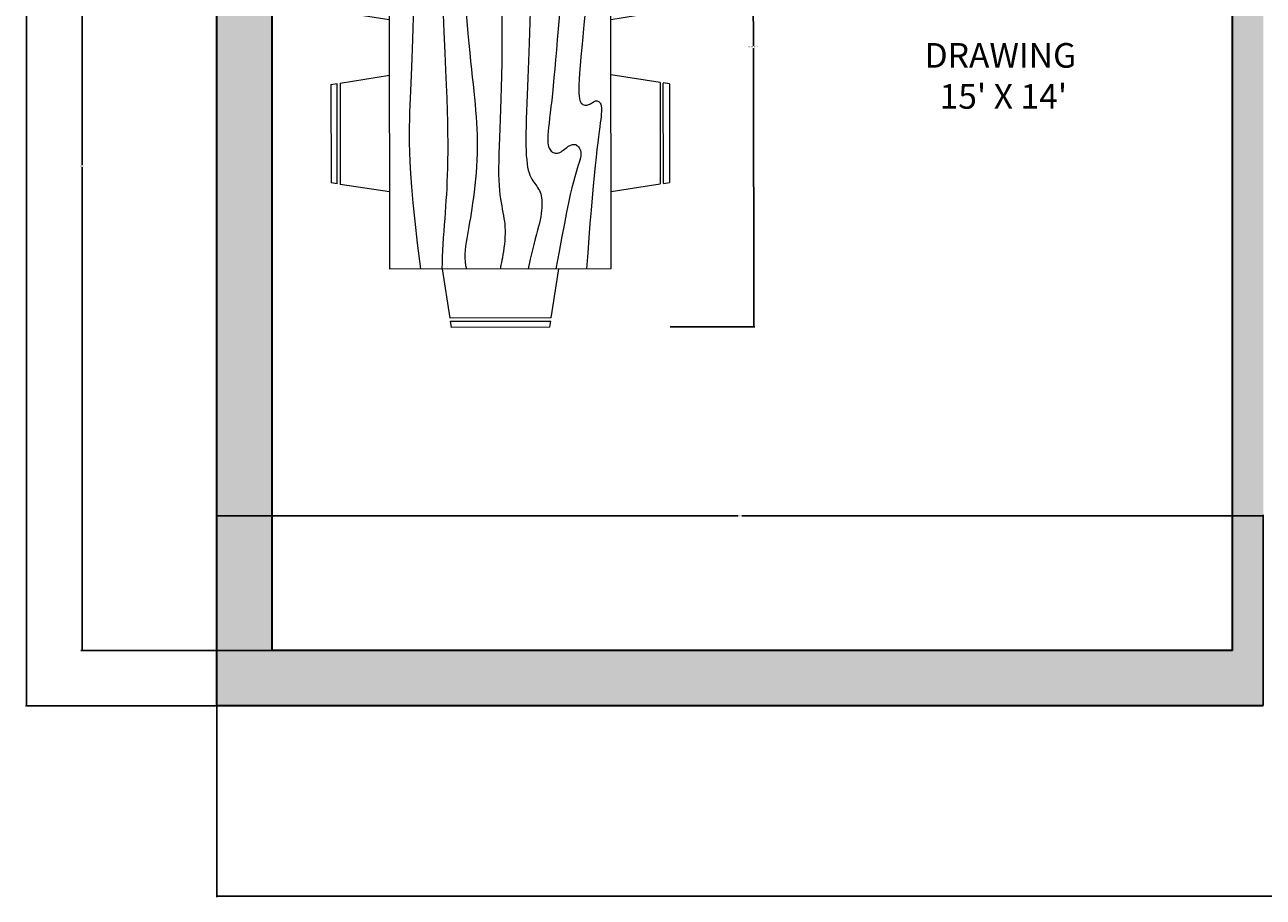
# Model space of a CAD drawing. Units: inches. Extents: x -30 to 437, y -29 to 647.
# Tile 1 of 15: x -30 to 172, y -29 to 113. Entities that reach past the tile are written whole.
import ezdxf

# ---------------------------------------------------------------- set-up
doc = ezdxf.new("R2010")
doc.units = ezdxf.units.IN
doc.header["$MEASUREMENT"] = 0
for name, color, linetype, lineweight in [('A-ANNO-DIMS', 2, 'Continuous', 18), ('A-AREA-IDEN', 7, 'Continuous', 18), ('A-WALL', 7, 'Continuous', 35), ('furniture', 220, 'Continuous', 18)]:
    doc.layers.add(name, color=color, linetype=linetype, lineweight=lineweight)
doc.layers.add('A-WALL-PATT', color=251, linetype='Continuous', lineweight=13, true_color=0x636466)
doc.styles.get("Standard").update_dxf_attribs({"font": 'arial.ttf'})
doc.dimstyles.get("Standard").update_dxf_attribs({"dimtxt": 0.18, "dimasz": 0.18, "dimexe": 0.18, "dimexo": 0.0625, "dimgap": 0.09, "dimtad": 0, "dimtih": 1, "dimtoh": 1, "dimdec": 4, "dimzin": 0, "dimdsep": 46, "dimtxsty": 'Standard', "dimcen": 0.09, "dimadec": 0, "dimazin": 0, "dimtfac": 1, "dimtdec": 4, "dimtofl": 0, "dimtmove": 0, "dimatfit": 3, "dimfxl": 1, "dimtolj": 1, "dimtzin": 0, "dimarcsym": 0})

# ---------------------------------------------------------------- blocks, each defined once
blk = doc.blocks.new('Dining Set - 36 x 72 in.')
for p, q in [((-22, 27.5), (-22.1562, 26.50042)), ((-5.8416, 26.5), (-22.1534, 26.5)), ((-22, 27.5), (-6, 27.5)), ((-5.8437, 26.49966), (-6, 27.5)), ((6, 27.5), (5.8438, 26.50042)), ((22.1584, 26.5), (5.8466, 26.5)), ((6, 27.5), (22, 27.5)), ((22.1563, 26.49966), (22, 27.5)), ((-22.2343, 26.00059), (-23.4847, 17.99762)), ((-22.2304, 26), (-5.7608, 26)), ((-4.5152, 17.99762), (-5.7655, 25.99926)), ((5.7657, 26.00059), (4.5153, 17.99762)), ((5.7696, 26), (22.2392, 26)), ((23.4848, 17.99762), (22.2345, 25.99926)), ((36, 18), (-36, 18)), ((-36, 18), (-36, -18)), ((36, -18), (36, 18)), ((-45.5, 8), (-44.5004, 8.15617)), ((-44.5, -8.15843), (-44.5, 8.15338)), ((-44.0006, 8.23428), (-35.9976, 9.48474)), ((-44, 8.23041), (-44, -8.23915)), ((44.0006, 8.23428), (35.9976, 9.48474)), ((44, 8.23041), (44, -8.23915)), ((44.5, -8.15843), (44.5, 8.15338)), ((45.5, 8), (44.5005, 8.15617)), ((-45.5, 8), (-45.5, -8)), ((45.5, 8), (45.5, -8)), ((-44.4997, -8.15631), (-45.5, -8)), ((44.4997, -8.15631), (45.5, -8)), ((-35.9976, -9.48476), (-43.9993, -8.2345)), ((35.9976, -9.48476), (43.9993, -8.2345)), ((-36, -18), (36, -18)), ((-22.2343, -26.0006), (-23.4847, -17.99762)), ((-4.5152, -17.99762), (-5.7655, -25.99928)), ((5.7657, -26.0006), (4.5153, -17.99762)), ((23.4848, -17.99762), (22.2345, -25.99928)), ((-22.2304, -26), (-5.7608, -26)), ((5.7696, -26), (22.2392, -26)), ((-22, -27.5), (-22.1562, -26.50044)), ((-5.8416, -26.5), (-22.1534, -26.5)), ((-22, -27.5), (-6, -27.5)), ((-5.8437, -26.49967), (-6, -27.5)), ((6, -27.5), (5.8438, -26.50044)), ((22.1584, -26.5), (5.8466, -26.5)), ((6, -27.5), (22, -27.5)), ((22.1563, -26.49967), (22, -27.5))]:
    blk.add_line(p, q)
for points in [[(-36, 15), (-31.1772, 14.97754), (-26.8079, 14.91406), (-22.8538, 14.81543), (-19.276, 14.6875), (-16.0362, 14.53613), (-13.0957, 14.36718), (-10.4159, 14.18652), (-7.9583, 14), (-5.6904, 13.81315), (-3.6035, 13.63021), (-1.6954, 13.45508), (0.0365, 13.29166), (1.5945, 13.14388), (2.9811, 13.01562), (4.1988, 12.9108), (5.25, 12.83333), (6.1393, 12.78613), (6.8802, 12.76823), (7.4883, 12.77767), (7.9792, 12.8125), (8.3685, 12.87077), (8.6719, 12.95052), (8.9049, 13.0498), (9.0833, 13.16666), (9.2205, 13.29899), (9.3216, 13.44401), (9.3895, 13.59879), (9.4271, 13.76041), (9.4373, 13.92594), (9.4232, 14.09245), (9.3875, 14.257), (9.3333, 14.41666), (9.2638, 14.56917), (9.1836, 14.71484), (9.0975, 14.85465), (9.0104, 14.98958), (8.9272, 15.1206), (8.8529, 15.2487), (8.7922, 15.37483), (8.75, 15.5), (8.7305, 15.62467), (8.7344, 15.74739), (8.7617, 15.86621), (8.8125, 15.97916), (8.8867, 16.08431), (8.9844, 16.17968), (9.1055, 16.26334), (9.25, 16.33333), (9.4189, 16.38802), (9.6172, 16.42708), (9.8506, 16.45052), (10.125, 16.45833), (10.4463, 16.45052), (10.8203, 16.42708), (11.2529, 16.38802), (11.75, 16.33333), (12.3184, 16.26318), (12.9694, 16.17838), (13.7151, 16.07991), (14.5677, 15.96875), (15.5395, 15.84586), (16.6426, 15.71224), (17.8893, 15.56884), (19.2917, 15.41666), (20.859, 15.25667), (22.5879, 15.08984), (24.4721, 14.91715), (26.5052, 14.73958), (28.6809, 14.5581), (30.9929, 14.3737), (33.4347, 14.18733), (36, 14)], [(-36, 10), (-28.9766, 10.14274), (-23.1725, 10.20442), (-18.4241, 10.19775), (-14.5677, 10.13541), (-11.4399, 10.03011), (-8.877, 9.89453), (-6.7154, 9.74137), (-4.7917, 9.58333), (-2.9698, 9.43082), (-1.2246, 9.28515), (0.4415, 9.14534), (2.026, 9.01041), (3.5266, 8.87939), (4.9408, 8.7513), (6.266, 8.62516), (7.5, 8.5), (8.6411, 8.37549), (9.6914, 8.2539), (10.6538, 8.13818), (11.5312, 8.03125), (12.3267, 7.93603), (13.043, 7.85547), (13.6831, 7.79248), (14.25, 7.75), (14.7471, 7.7303), (15.1797, 7.73307), (15.5537, 7.75732), (15.875, 7.80208), (16.1494, 7.86637), (16.3828, 7.94922), (16.5811, 8.04964), (16.75, 8.16666), (16.8944, 8.29915), (17.0143, 8.44531), (17.1089, 8.60319), (17.1771, 8.77083), (17.218, 8.94629), (17.2305, 9.1276), (17.2137, 9.31282), (17.1667, 9.5), (17.0895, 9.6875), (16.987, 9.875), (16.8649, 10.0625), (16.7292, 10.25), (16.5856, 10.4375), (16.4401, 10.625), (16.2985, 10.8125), (16.1667, 11), (16.05, 11.18733), (15.9518, 11.3737), (15.8752, 11.5581), (15.8229, 11.73958), (15.798, 11.91715), (15.8034, 12.08984), (15.842, 12.25667), (15.9167, 12.41666), (16.0295, 12.56836), (16.1784, 12.70833), (16.3605, 12.83268), (16.5729, 12.9375), (16.8127, 13.01888), (17.0768, 13.07291), (17.3625, 13.0957), (17.6667, 13.08333), (17.9894, 13.03312), (18.3418, 12.94726), (18.7382, 12.82918), (19.1927, 12.68229), (19.7195, 12.51001), (20.3327, 12.31575), (21.0465, 12.10294), (21.875, 11.875), (22.8357, 11.63354), (23.959, 11.37304), (25.2786, 11.08618), (26.8282, 10.76562), (28.6414, 10.40405), (30.752, 9.99414), (33.1936, 9.52856), (36, 9)], [(-36, 5.5), (-30.7157, 5.3348), (-26.069, 5.20963), (-21.9946, 5.11767), (-18.4271, 5.05208), (-15.3009, 5.00602), (-12.5508, 4.97265), (-10.1112, 4.94515), (-7.9167, 4.91666), (-5.909, 4.88167), (-4.0586, 4.83984), (-2.3429, 4.79215), (-0.7396, 4.73958), (0.7739, 4.6831), (2.22, 4.6237), (3.6213, 4.56233), (5, 4.5), (6.373, 4.43782), (7.7344, 4.3776), (9.0723, 4.32129), (10.375, 4.27083), (11.6309, 4.22819), (12.8281, 4.19531), (13.9551, 4.17415), (15, 4.16666), (15.954, 4.17448), (16.819, 4.19791), (17.6001, 4.23698), (18.3021, 4.29166), (18.9299, 4.36198), (19.4883, 4.44791), (19.9823, 4.54948), (20.4167, 4.66666), (20.7969, 4.79899), (21.1302, 4.94401), (21.4245, 5.09879), (21.6875, 5.26041), (21.9271, 5.42594), (22.1511, 5.59245), (22.3672, 5.757), (22.5834, 5.91666), (22.8065, 6.06868), (23.0404, 6.21093), (23.2879, 6.34147), (23.5521, 6.45833), (23.8358, 6.55957), (24.142, 6.64323), (24.4735, 6.70735), (24.8334, 6.75), (25.2235, 6.76969), (25.642, 6.76692), (26.0858, 6.74267), (26.5521, 6.69791), (27.0379, 6.63362), (27.5404, 6.55078), (28.0565, 6.45036), (28.5834, 6.33333), (29.1242, 6.19987), (29.7071, 6.04687), (30.3661, 5.87044), (31.1354, 5.66666), (32.0493, 5.43164), (33.142, 5.16146), (34.4475, 4.85221), (36, 4.5)], [(-36, -1), (-30.7915, -0.6591), (-26.0195, -0.38216), (-21.6519, -0.16284), (-17.6563, 0.00521), (-14.0005, 0.12833), (-10.6523, 0.21289), (-7.5796, 0.26522), (-4.75, 0.29166), (-2.134, 0.29793), (0.2878, 0.28711), (2.5317, 0.26163), (4.6146, 0.22396), (6.5529, 0.17651), (8.3633, 0.12174), (10.0623, 0.06209), (11.6667, 0), (13.1899, -0.06201), (14.6341, -0.1211), (15.9982, -0.17432), (17.2813, -0.21875), (18.4823, -0.25147), (19.6003, -0.26953), (20.6343, -0.27002), (21.5834, -0.25), (22.4481, -0.20768), (23.2357, -0.14584), (23.9549, -0.06836), (24.6146, 0.02083), (25.2235, 0.11784), (25.7904, 0.21875), (26.3241, 0.31966), (26.8334, 0.41666), (27.3265, 0.50618), (27.8099, 0.58593), (28.2894, 0.65397), (28.7709, 0.70833), (29.2601, 0.74707), (29.763, 0.76823), (30.2855, 0.76985), (30.8334, 0.75), (31.4088, 0.70784), (31.9994, 0.64713), (32.589, 0.57275), (33.1615, 0.48958), (33.7008, 0.4025), (34.1908, 0.3164), (34.6153, 0.23616), (34.9584, 0.16666), (35.2099, 0.11165), (35.3848, 0.07031), (35.504, 0.04069), (35.5886, 0.02083), (35.6594, 0.00879), (35.7377, 0.0026), (35.8442, 0.00032), (36, 0)], [(-36, -6.5), (-27.1843, -6.31267), (-20.084, -6.1263), (-14.469, -5.9419), (-10.1094, -5.76042), (-6.7752, -5.58285), (-4.2363, -5.41016), (-2.2629, -5.24333), (-0.625, -5.08334), (0.8708, -4.93099), (2.2715, -4.78646), (3.5872, -4.64974), (4.8281, -4.52084), (6.0046, -4.39974), (7.127, -4.28646), (8.2053, -4.18099), (9.25, -4.08334), (10.2705, -3.99382), (11.2734, -3.91407), (12.2647, -3.84603), (13.25, -3.79167), (14.2354, -3.75293), (15.2266, -3.73177), (16.2295, -3.73015), (17.25, -3.75), (18.2912, -3.79248), (19.3451, -3.85547), (20.4009, -3.93604), (21.4479, -4.03125), (22.4754, -4.13819), (23.4727, -4.25391), (24.4289, -4.37549), (25.3334, -4.5), (26.1785, -4.62492), (26.9694, -4.74935), (27.7145, -4.87281), (28.4219, -4.99479), (29.1, -5.11483), (29.7572, -5.23242), (30.4016, -5.34709), (31.0417, -5.45834), (31.6837, -5.56437), (32.3262, -5.65821), (32.9658, -5.73153), (33.599, -5.77604), (34.2224, -5.78345), (34.8327, -5.74545), (35.4264, -5.65373), (36, -5.5)], [(-36, -10), (-26.4022, -9.81299), (-18.4675, -9.62891), (-11.9839, -9.45069), (-6.7396, -9.28125), (-2.5226, -9.12354), (0.8789, -8.98047), (3.6769, -8.85498), (6.0833, -8.75), (8.2767, -8.66765), (10.3021, -8.60677), (12.1712, -8.56543), (13.8958, -8.54167), (15.4876, -8.53353), (16.9583, -8.53907), (18.3197, -8.55632), (19.5834, -8.58334), (20.7616, -8.61841), (21.8685, -8.66081), (22.9188, -8.71004), (23.9271, -8.76563), (24.9081, -8.82707), (25.8763, -8.89388), (26.8465, -8.96558), (27.8334, -9.04167), (28.8474, -9.12118), (29.8828, -9.20117), (30.93, -9.27824), (31.9792, -9.34896), (33.0205, -9.40991), (34.0443, -9.45768), (35.0407, -9.48885), (36, -9.5)], [(-36, -14.5), (-30.0881, -14.33513), (-25.0332, -14.21224), (-20.7312, -14.12647), (-17.0781, -14.07292), (-13.97, -14.04671), (-11.3027, -14.04297), (-8.9724, -14.05681), (-6.875, -14.08334), (-4.9224, -14.11833), (-3.0905, -14.16016), (-1.3709, -14.20785), (0.2448, -14.26042), (1.7647, -14.3169), (3.1973, -14.3763), (4.5507, -14.43767), (5.8333, -14.5), (7.0554, -14.5621), (8.235, -14.62175), (9.3922, -14.67652), (10.5469, -14.72396), (11.7192, -14.76164), (12.929, -14.78711), (14.1965, -14.79794), (15.5417, -14.79167), (16.9933, -14.76424), (18.6152, -14.70508), (20.4804, -14.60197), (22.6615, -14.44271), (25.2312, -14.21509), (28.2624, -13.9069), (31.8277, -13.50594), (36, -13)]]:
    blk.add_lwpolyline(points)
blk = doc.blocks.new('*D19')
at = {"layer": 'A-ANNO-DIMS', "color": 0, "lineweight": -2, "transparency": 16777216}
for p, q in [((75.18, 154.64), (88.95, 154.66)), ((88.77, 154.48), (88.84, 109.34)), ((88.91, 63.84), (88.84, 108.98)), ((75.32, 63.64), (89.09, 63.66))]:
    blk.add_line(p, q, dxfattribs=at)
at = {"layer": 'A-ANNO-DIMS', "color": 0, "transparency": 16777216}
for points in [[(88.8, 154.48), (88.74, 154.48), (88.77, 154.66)], [(88.94, 63.84), (88.88, 63.84), (88.91, 63.66)]]:
    blk.add_solid(points, dxfattribs=at)
at = {"layer": 'Defpoints', "color": 0, "transparency": 16777216}
for p in [(75.12, 154.64), (75.26, 63.64), (88.91, 63.66)]:
    blk.add_point(p, dxfattribs=at)
at = {"layer": 'A-ANNO-DIMS', "color": 0, "transparency": 16777216, "insert": (88.84, 109.16), "char_height": 0.18, "attachment_point": 5}
blk.add_mtext('\\A1;DINING SET 91', dxfattribs=at)
blk = doc.blocks.new('*D25')
at = {"layer": 'A-ANNO-DIMS', "color": 0, "lineweight": -2, "transparency": 16777216}
for p, q in [((1.67, 1.98), (1.67, -29.03)), ((405.67, 1.98), (405.67, -29.03)), ((1.85, -28.85), (203.38, -28.85)), ((405.49, -28.85), (203.97, -28.85))]:
    blk.add_line(p, q, dxfattribs=at)
at = {"layer": 'A-ANNO-DIMS', "color": 0, "transparency": 16777216}
for points in [[(1.85, -28.82), (1.85, -28.88), (1.67, -28.85)], [(405.49, -28.82), (405.49, -28.88), (405.67, -28.85)]]:
    blk.add_solid(points, dxfattribs=at)
at = {"layer": 'Defpoints', "color": 0, "transparency": 16777216}
for p in [(1.67, 2.05), (405.67, 2.05), (405.67, -28.85)]:
    blk.add_point(p, dxfattribs=at)
at = {"layer": 'A-ANNO-DIMS', "color": 0, "transparency": 16777216, "insert": (203.67, -28.85), "char_height": 0.18, "attachment_point": 5}
blk.add_mtext('\\A1;404', dxfattribs=at)
blk = doc.blocks.new('*D26')
at = {"layer": 'A-ANNO-DIMS', "color": 0, "lineweight": -2, "transparency": 16777216}
for p, q in [((1.61, 615.55), (-29.41, 615.55)), ((-29.23, 615.37), (-29.23, 308.98)), ((-29.23, 2.23), (-29.23, 308.62)), ((1.61, 2.05), (-29.41, 2.05))]:
    blk.add_line(p, q, dxfattribs=at)
at = {"layer": 'A-ANNO-DIMS', "color": 0, "transparency": 16777216}
for points in [[(-29.26, 615.37), (-29.2, 615.37), (-29.23, 615.55)], [(-29.26, 2.23), (-29.2, 2.23), (-29.23, 2.05)]]:
    blk.add_solid(points, dxfattribs=at)
at = {"layer": 'Defpoints', "color": 0, "transparency": 16777216}
for p in [(-29.23, 615.55), (1.67, 615.55), (1.67, 2.05)]:
    blk.add_point(p, dxfattribs=at)
at = {"layer": 'A-ANNO-DIMS', "color": 0, "transparency": 16777216, "insert": (-29.23, 308.8), "char_height": 0.18, "attachment_point": 5}
blk.add_mtext('\\A1;613.5', dxfattribs=at)
blk = doc.blocks.new('*D30')
at = {"layer": 'A-ANNO-DIMS', "color": 0, "lineweight": -2, "transparency": 16777216}
for p, q in [((10.61, 168.55), (-20.41, 168.55)), ((-20.23, 168.37), (-20.23, 89.98)), ((-20.23, 11.23), (-20.23, 89.62)), ((10.61, 11.05), (-20.41, 11.05))]:
    blk.add_line(p, q, dxfattribs=at)
at = {"layer": 'A-ANNO-DIMS', "color": 0, "transparency": 16777216}
for points in [[(-20.26, 168.37), (-20.2, 168.37), (-20.23, 168.55)], [(-20.26, 11.23), (-20.2, 11.23), (-20.23, 11.05)]]:
    blk.add_solid(points, dxfattribs=at)
at = {"layer": 'Defpoints', "color": 0, "transparency": 16777216}
for p in [(-20.23, 168.55), (10.67, 168.55), (10.67, 11.05)]:
    blk.add_point(p, dxfattribs=at)
at = {"layer": 'A-ANNO-DIMS', "color": 0, "transparency": 16777216, "insert": (-20.23, 89.8), "char_height": 0.18, "attachment_point": 5}
blk.add_mtext('\\A1;157.5', dxfattribs=at)
blk = doc.blocks.new('*D35')
at = {"layer": 'A-ANNO-DIMS', "color": 0, "lineweight": -2, "transparency": 16777216}
for p, q in [((1.67, 2.11), (1.67, 33.13)), ((1.85, 32.95), (86.39, 32.95)), ((171.49, 32.95), (86.95, 32.95)), ((171.67, 2.11), (171.67, 33.13))]:
    blk.add_line(p, q, dxfattribs=at)
at = {"layer": 'A-ANNO-DIMS', "color": 0, "transparency": 16777216}
for points in [[(1.85, 32.98), (1.85, 32.92), (1.67, 32.95)], [(171.49, 32.98), (171.49, 32.92), (171.67, 32.95)]]:
    blk.add_solid(points, dxfattribs=at)
at = {"layer": 'Defpoints', "color": 0, "transparency": 16777216}
for p in [(171.67, 32.95), (1.67, 2.05), (171.67, 2.05)]:
    blk.add_point(p, dxfattribs=at)
at = {"layer": 'A-ANNO-DIMS', "color": 0, "transparency": 16777216, "insert": (86.67, 32.95), "char_height": 0.18, "attachment_point": 5}
blk.add_mtext('\\A1;170', dxfattribs=at)

msp = doc.modelspace()

# ---------------------------------------------------------------- hatches: boundary and pattern name
at = {"layer": 'A-WALL-PATT'}
h = msp.add_hatch(color=256, dxfattribs=at)
h.dxf.hatch_style = 1
h.paths.add_polyline_path([(393.6054, 183.2352), (369.6054, 183.2352), (369.6054, 213.2352), (393.6054, 213.2352), (393.6054, 207.2352), (394.6054, 207.2352), (394.6054, 211.2352), (395.6054, 211.2352), (395.6054, 185.2352), (394.6054, 185.2352), (394.6054, 189.2352), (393.6054, 189.2352)], flags=0)
h.paths.add_polyline_path([(384.6054, 189.2352, -1), (390.6054, 189.2352, -1)], flags=0)
h.paths.add_polyline_path([(385.6054, 189.2352, -1), (389.6054, 189.2352, -1)], flags=0)
h.paths.add_polyline_path([(374.6054, 189.2352, -1), (382.6054, 189.2352, -1)], flags=0)
h.paths.add_polyline_path([(386.6054, 189.2352, -1), (388.6054, 189.2352, -1)], flags=0)
h.paths.add_polyline_path([(375.6054, 189.2352, -1), (381.6054, 189.2352, -1)], flags=0)
h.paths.add_polyline_path([(376.6054, 189.2352, -1), (380.6054, 189.2352, -1)], flags=0)
h.paths.add_polyline_path([(377.6054, 189.2352, -1), (379.6054, 189.2352, -1)], flags=0)
h.paths.add_polyline_path([(390.6054, 195.2352), (374.6054, 195.2352), (374.6054, 201.2352), (390.6054, 201.2352)], flags=0)
h.paths.add_polyline_path([(389.6054, 196.2352), (375.6054, 196.2352), (375.6054, 200.2352), (389.6054, 200.2352)], flags=0)
h.paths.add_polyline_path([(383.6054, 207.2352, -1), (391.6054, 207.2352, -1)], flags=0)
h.paths.add_polyline_path([(384.6054, 207.2352, -1), (390.6054, 207.2352, -1)], flags=0)
h.paths.add_polyline_path([(385.6054, 207.2352, -1), (389.6054, 207.2352, -1)], flags=0)
h.paths.add_polyline_path([(386.6054, 207.2352, -1), (388.6054, 207.2352, -1)], flags=0)
h.paths.add_polyline_path([(375.6054, 207.2352, -1), (381.6054, 207.2352, -1)], flags=0)
h.paths.add_polyline_path([(376.6054, 207.2352, -1), (380.6054, 207.2352, -1)], flags=0)
h.paths.add_polyline_path([(377.6054, 207.2352, -1), (379.6054, 207.2352, -1)], flags=0)
h.paths.add_polyline_path([(305.5437, 160.3663, -0.41421356), (304.0437, 158.8663), (271.0437, 158.8663, -0.41421356), (269.5437, 160.3663), (269.5437, 178.3663, -0.41421356), (271.0437, 179.8663), (304.0437, 179.8663, -0.41421356), (305.5437, 178.3663)], flags=0)
h.paths.add_polyline_path([(304.0437, 165.3663, -0.41421356), (303.0437, 164.3663), (289.2937, 164.3663, -0.41421356), (288.2937, 165.3663), (288.2937, 177.3663, -0.41421356), (289.2937, 178.3663), (303.0437, 178.3663, -0.41421356), (304.0437, 177.3663)], flags=0)
h.paths.add_polyline_path([(296.5437, 171.3663, -1), (295.5437, 171.3663, -1)], flags=0)
h.paths.add_polyline_path([(286.7937, 165.3663, -0.41421356), (285.7937, 164.3663), (272.0437, 164.3663, -0.41421356), (271.0437, 165.3663), (271.0437, 177.3663, -0.41421356), (272.0437, 178.3663), (285.7937, 178.3663, -0.41421356), (286.7937, 177.3663)], flags=0)
h.paths.add_polyline_path([(279.5437, 171.3663, -1), (278.5437, 171.3663, -1)], flags=0)
h.paths.add_polyline_path([(360.6737, 290.5474), (360.6737, 300.5474), (396.6737, 300.5474), (396.6737, 290.5474)], flags=0)
h.paths.add_polyline_path([(259.6737, 124.5474), (259.6737, 114.5474), (171.6737, 114.5474), (171.6737, 124.5474)], flags=0)
h.paths.add_polyline_path([(288.0737, 215.3705), (286.7097, 214.583), (268.7097, 245.7599), (270.0737, 246.5474)], flags=0)
h.paths.add_polyline_path([(259.6737, 168.5474), (256.6737, 168.5474), (256.6737, 173.5474), (256.6737, 179.0224), (255.8753, 177.6395), (224.2956, 195.872, 0.12053744), (220.1737, 179.0224, 0.12053744), (216.0518, 195.872), (184.4721, 177.6395), (183.6737, 179.0224), (215.2836, 197.2724), (216.0821, 195.8895), (216.0518, 195.872, -0.12053744), (220.1737, 179.0224, -0.12053744), (224.2956, 195.872), (224.2653, 195.8895), (225.0638, 197.2724), (256.6737, 179.0224), (256.6737, 173.5474), (259.6737, 173.5474)], flags=0)
h.paths.add_polyline_path([(386.7943, 325.4601), (372.6871, 325.4601), (372.6871, 339.5673), (386.7943, 339.5673)], flags=0)
h.paths.add_polyline_path([(359.5875, 343.7429), (357.7905, 343.7429), (357.7905, 327.9179), (359.3933, 327.9179, 0.41420885), (361.5302, 330.0549), (361.5302, 341.8434, 0.41436161)], flags=0)
h.paths.add_polyline_path([(341.7887, 323.1235, -0.11921667), (340.7839, 323.1235)], flags=0)
h.paths.add_polyline_path([(379.6332, 328.8632), (379.6332, 332.2699), (376.0992, 332.2699, 0.39427733)], flags=0)
h.paths.add_polyline_path([(375.5299, 332.459, -1), (383.8511, 332.459, -1)], flags=0)
h.paths.add_polyline_path([(388.9363, 344.7425), (372.5309, 344.7425, -0.41421356), (370.394, 346.8794), (370.394, 347.5594, -0.39085173), (372.3472, 349.7005, -0.43951011), (370.394, 351.4933), (370.394, 365.1894, -0.40305452), (372.2191, 367.1298, -0.41839453), (370.394, 368.9291), (370.394, 382.6251, -0.40885826), (372.2519, 384.5722, -0.42377324), (370.394, 386.3707), (370.394, 400.0667, -0.38660687), (372.1327, 402.0094), (372.531, 402.0094, -0.41421834), (370.394, 404.1464), (370.394, 404.7778, -0.41420891), (372.5309, 406.9147), (388.9363, 406.9147, -0.41421821), (391.0733, 404.7778), (391.0733, 346.8794, -0.41421356)], flags=0)
edge = h.paths.add_edge_path(flags=0)
edge.add_spline(control_points=[(349.3585, 363.204), (349.0859, 363.204), (348.8133, 363.2227), (348.2712, 363.2973), (348.0016, 363.3531), (347.3533, 363.5328), (346.9776, 363.6755), (346.2445, 364.0308), (345.887, 364.2432), (345.1953, 364.7329), (344.8611, 365.0101), (344.2197, 365.6237), (343.9125, 365.9603), (343.211, 366.8336), (342.8313, 367.3965), (342.1401, 368.6117), (341.8286, 369.2641), (341.2807, 370.64), (341.0443, 371.3636), (340.6522, 372.8619), (340.4964, 373.6367), (340.2695, 375.2158), (340.1983, 376.0203), (340.142, 377.6365), (340.157, 378.4483), (340.2729, 380.0567), (340.3738, 380.8533), (340.6589, 382.4093), (340.8432, 383.1686), (341.2906, 384.629), (341.5538, 385.3301), (342.1531, 386.6544), (342.4891, 387.2776), (343.2266, 388.4288), (343.6281, 388.9567), (344.4879, 389.9012), (344.9463, 390.3178), (345.7981, 390.9428), (346.182, 391.1771), (346.9712, 391.5648), (347.3766, 391.7182), (348.2004, 391.9387), (348.6189, 392.0058), (349.4588, 392.0508), (349.8801, 392.0288), (350.7146, 391.8966), (351.1278, 391.7865), (351.9366, 391.4822), (352.3323, 391.2882), (353.0989, 390.8223), (353.4699, 390.5504), (354.1819, 389.9355), (354.5229, 389.5924), (355.1706, 388.8418), (355.4772, 388.4343), (356.1315, 387.4422), (356.4671, 386.8397), (357.0692, 385.5581), (357.3356, 384.879), (357.7933, 383.4624), (357.9846, 382.725), (358.2875, 381.2112), (358.3992, 380.4349), (358.5404, 378.8643), (358.5699, 378.0699), (358.546, 376.4841), (358.4926, 375.6928), (358.3042, 374.1343), (358.1692, 373.3672), (357.8207, 371.8774), (357.6072, 371.1549), (357.1067, 369.7735), (356.8196, 369.1148), (356.1782, 367.8787), (355.8238, 367.3013), (355.0551, 366.244), (354.6408, 365.7641), (353.7607, 364.9161), (353.2948, 364.5481), (352.445, 364.0149), (352.0701, 363.822), (351.3034, 363.5117), (350.9116, 363.3943), (350.1325, 363.2418), (349.7455, 363.204), (349.3585, 363.204)], knot_values=[3.14159265, 3.14159265, 3.14159265, 3.14159265, 3.22691715, 3.22691715, 3.31224165, 3.31224165, 3.43426671, 3.43426671, 3.55629177, 3.55629177, 3.67831683, 3.67831683, 3.8003419, 3.8003419, 3.97157384, 3.97157384, 4.14280577, 4.14280577, 4.31403771, 4.31403771, 4.48526965, 4.48526965, 4.65650159, 4.65650159, 4.82773353, 4.82773353, 4.99896547, 4.99896547, 5.1701974, 5.1701974, 5.34142934, 5.34142934, 5.51266128, 5.51266128, 5.68389322, 5.68389322, 5.85512516, 5.85512516, 5.98669107, 5.98669107, 6.11825699, 6.11825699, 6.24982291, 6.24982291, 6.38138882, 6.38138882, 6.51295474, 6.51295474, 6.64452065, 6.64452065, 6.77608657, 6.77608657, 6.90765249, 6.90765249, 7.0392184, 7.0392184, 7.20701563, 7.20701563, 7.37481286, 7.37481286, 7.54261009, 7.54261009, 7.71040732, 7.71040732, 7.87820455, 7.87820455, 8.04600178, 8.04600178, 8.21379901, 8.21379901, 8.38159624, 8.38159624, 8.54939347, 8.54939347, 8.7171907, 8.7171907, 8.88498794, 8.88498794, 9.05278517, 9.05278517, 9.17820699, 9.17820699, 9.30362881, 9.30362881, 9.42477796, 9.42477796, 9.42477796, 9.42477796], degree=3, periodic=0)
edge.add_line((341.1696, 384.3006), (341.2012, 384.2808))
edge = h.paths.add_edge_path(flags=0)
edge.add_line((344.3353, 388.7801), (344.317, 388.7915))
edge.add_ellipse((349.3585, 377.6204), major_axis=(0, -13.7895), ratio=0.62186025, start_angle=-244.867444, end_angle=-124.769923)
h.paths.add_polyline_path([(163.6737, 163.1474), (132.4968, 145.1474), (131.7093, 146.5114), (162.8862, 164.5114)], flags=0)
h.paths.add_polyline_path([(366.4355, 409.0896, -0.41423669), (364.2985, 406.9525, -0.4913499), (361.5302, 408.8973), (361.5302, 420.6405, 0.41421356), (359.3932, 422.7775), (357.7905, 422.7775), (357.7905, 406.9525), (359.6317, 406.9525, 0.42741026), (361.5332, 408.9757, 0.39869469), (363.6672, 406.9525, 0.51958103), (366.4355, 409.0895)], flags=0)
h.paths.add_polyline_path([(386.7943, 410.9671), (372.6871, 410.9671), (372.6871, 425.0742), (386.7943, 425.0742)], flags=0)
h.paths.add_polyline_path([(379.6332, 414.3701), (379.6332, 417.7768), (376.0992, 417.7768, 0.39427733)], flags=0)
h.paths.add_polyline_path([(375.5299, 417.966, -1), (383.8511, 417.966, -1)], flags=0)
h.paths.add_polyline_path([(150.0377, 351.583), (148.6737, 352.3705), (166.6737, 383.5474), (168.0377, 382.7599)], flags=0)
h.paths.add_polyline_path([(91.6737, 234.1974), (66.559, 219.6974), (65.9246, 220.7962), (91.0393, 235.2962)], flags=0)
h.paths.add_polyline_path([(255.4612, 443.5834), (254.6737, 444.9474), (285.8506, 462.9474), (286.6381, 461.5834)], flags=0)
h.paths.add_polyline_path([(176.2737, 394.5474), (158.2737, 425.7243), (159.6377, 426.5118), (177.6377, 395.3349)], flags=0)
h.paths.add_polyline_path([(243.6737, 439.5474), (243.0393, 438.4486), (217.9246, 452.9486), (218.559, 454.0474)], flags=0)
h.paths.add_polyline_path([(38.1264, 269.8429), (40.2408, 269.8429), (40.2408, 270.3508), (38.1264, 270.3508)], flags=0)
h.paths.add_polyline_path([(75.7157, 289.9439), (40.2408, 289.9439), (38.1264, 289.6524), (40.2408, 289.6524)], flags=0)
h.paths.add_polyline_path([(75.7157, 270.0846), (77.6447, 270.0846), (77.6697, 270.1626), (75.7175, 270.1626)], flags=0)
h.paths.add_polyline_path([(80.5373, 293.3002), (33.0467, 293.3002), (13.5054, 293.3002), (13.5054, 351.9244), (29.7898, 351.9244), (80.5373, 351.9244)], flags=0)
h.paths.add_polyline_path([(46.0261, 212.466, -0.50131678), (27.1651, 207.5106), (21.165, 209.5107), (21.165, 206.5107), (22.665, 206.5107), (22.665, 203.5107), (21.165, 203.5107), (21.165, 203.0107), (13.165, 203.0107), (13.165, 224.0107), (21.165, 224.0107), (21.165, 217.5107), (27.1649, 219.5106, -0.50132349), (46.0261, 214.5554, -0.13289091)], flags=0)
h.paths.add_polyline_path([(44.688, 211.8666, -0.48007965), (27.165, 209.5107), (27.165, 217.5107, -0.4800795), (44.688, 215.1547, -0.21500378)], flags=0)
h.paths.add_polyline_path([(19.415, 204.0107), (15.165, 204.0107, -0.41421356), (14.165, 204.7607), (14.165, 222.0107, -0.41421356), (14.915, 223.0107), (19.165, 223.0107, -0.41421356), (20.165, 222.2607), (20.165, 205.0107, -0.41421356)], flags=0)
h.paths.add_polyline_path([(32.7608, 269.0719), (31.8439, 269.0719), (31.8439, 268.6134), (13.5054, 268.6134), (13.5054, 291.5366), (31.8439, 291.5366), (32.7608, 291.0781), (32.7608, 280.9919, -1), (32.7608, 279.1581)], flags=0)
h.paths.add_polyline_path([(40.2408, 360.1436), (38.1264, 360.1436), (38.1264, 359.6357), (40.2408, 359.6357)], flags=0)
h.paths.add_polyline_path([(75.7157, 355.2807), (40.2408, 355.2807), (38.1264, 355.5722), (40.2408, 355.5722), (40.2408, 355.2807), (75.7157, 355.2807), (75.7157, 375.5982), (40.2408, 375.5982), (38.1264, 375.3817), (40.2408, 375.3817), (40.2408, 375.5982), (75.7157, 375.5982), (77.9733, 375.062), (75.7175, 375.062), (75.7175, 374.554)], flags=0)
h.paths.add_polyline_path([(42.8174, 299.814, 0.13867074), (34.1602, 294.603), (14.8081, 294.603), (14.8081, 350.6216), (29.8539, 350.6216, 0.09822056)], flags=0)
h.paths.add_polyline_path([(15.8636, 276.7781, -0.30640166), (20.3757, 283.4499), (20.3483, 290.6726), (31.4014, 290.7146), (31.4309, 282.9124), (26.8287, 282.895, -0.26006276), (30.241, 276.7781, -1)], flags=0)
h.paths.add_polyline_path([(26.1332, 276.7781), (23.0523, 273.6972), (19.9714, 276.7781), (23.0523, 279.8589), (23.0523, 283.9209), (21.3493, 283.9145), (20.7006, 283.5219), (20.6907, 286.1226), (23.2914, 286.1325), (25.8936, 285.7522), (27.1939, 285.7572), (28.4928, 286.1522), (31.0935, 286.1621), (31.0918, 286.6172), (25.6303, 286.5965), (25.616, 290.3675), (31.0775, 290.3882), (31.0918, 286.6172), (31.1034, 283.5614), (28.5027, 283.5515), (25.9005, 283.9317), (23.0523, 283.9209), (23.0523, 279.8589)], flags=0)
h.paths.add_polyline_path([(24.0793, 276.7781, -1), (22.0253, 276.7781, -1)], flags=0)
h.paths.add_polyline_path([(35.7687, 302.2895, -0.41421356), (35.2283, 301.2726), (22.2164, 297.2909, -0.41421356), (21.1995, 297.8313), (15.7317, 315.6996, -0.41421356), (16.2721, 316.7165), (18.8554, 317.507), (15.3721, 328.8904, -0.41421356), (15.9125, 329.9073), (28.9244, 333.889, -0.41421356), (29.9414, 333.3486), (35.4091, 315.4802, -0.41421356), (34.8687, 314.4633), (32.2854, 313.6728)], flags=0)
h.paths.add_polyline_path([(361.3728, 532.6207), (302.7487, 532.6207), (302.7487, 580.1113), (302.7487, 599.6527), (361.3728, 599.6527), (361.3728, 583.3682)], flags=0)
h.paths.add_polyline_path([(370.1, 575.0316), (370.1, 572.9172), (370.6079, 572.9172), (370.6079, 575.0316)], flags=0)
h.paths.add_polyline_path([(385.0466, 537.4423), (385.0466, 572.9172), (384.8302, 575.0316), (384.8302, 572.9172)], flags=0)
h.paths.add_polyline_path([(384.5104, 535.3262), (384.5104, 537.4406), (384.0025, 537.4406), (364.7291, 537.4423), (364.7291, 572.9172), (365.0206, 575.0316), (365.0206, 572.9172), (364.7291, 572.9172), (364.7291, 537.4423), (384.5884, 537.4423), (384.5884, 535.5133)], flags=0)
h.paths.add_polyline_path([(384.5884, 535.5133), (383.4945, 535.164), (383.4945, 537.4406), (382.9866, 535.3262), (382.9866, 537.4406), (383.4945, 535.3262), (383.4945, 537.4406), (384.5884, 537.4406)], flags=0)
h.paths.add_polyline_path([(23.874, 286.8174), (21.0132, 286.8065), (21.0004, 290.1875), (23.8612, 290.1983)], flags=0)
h.paths.add_polyline_path([(242.9824, 511.1667), (234.9824, 511.1667), (234.9824, 517.6667), (228.9825, 515.6667, -0.50132349), (210.1213, 520.622, -0.13289091), (210.1213, 522.7114, -0.50131678), (228.9823, 527.6667), (234.9824, 525.6667), (234.9824, 528.6667), (233.4824, 528.6667), (233.4824, 531.6667), (234.9824, 531.6667), (234.9824, 532.1667), (242.9824, 532.1667)], flags=0)
h.paths.add_polyline_path([(236.9824, 512.1667, -0.41421356), (235.9824, 512.9167), (235.9824, 530.1667, -0.41421356), (236.7324, 531.1667), (240.9824, 531.1667, -0.41421356), (241.9824, 530.4167), (241.9824, 513.1667, -0.41421356), (241.2324, 512.1667)], flags=0)
h.paths.add_polyline_path([(279.533, 537.4423), (279.533, 535.5133), (279.6111, 535.4884), (279.6111, 537.4406)], flags=0)
h.paths.add_polyline_path([(279.2913, 575.0316), (279.2913, 572.9172), (279.7992, 572.9172), (279.7992, 575.0316)], flags=0)
h.paths.add_polyline_path([(211.4594, 520.0227, -0.21500378), (211.4594, 523.3107, -0.48007965), (228.9824, 525.6667), (228.9824, 517.6667, -0.4800795)], flags=0)
h.paths.add_polyline_path([(32.7627, 354.1465), (31.8457, 354.1465), (31.8457, 353.688), (13.5054, 353.688), (13.5054, 376.6134), (31.8457, 376.6134), (32.7627, 376.1549), (32.7627, 366.0677, -1), (32.7627, 364.2337)], flags=0)
h.paths.add_polyline_path([(15.9446, 365.1507, -1), (30.3234, 365.1507, -1)], flags=0)
h.paths.add_polyline_path([(41.213, 428.467), (43.3274, 428.467), (43.3274, 428.9749), (41.213, 428.9749)], flags=0)
h.paths.add_polyline_path([(78.8022, 448.568), (43.3274, 448.568), (41.213, 448.2765), (43.3274, 448.2765)], flags=0)
h.paths.add_polyline_path([(78.8022, 428.7087), (80.7313, 428.7087), (80.7562, 428.7868), (78.804, 428.7868)], flags=0)
h.paths.add_polyline_path([(26.2152, 365.1507), (23.134, 362.0696), (20.0529, 365.1507), (23.134, 368.2319)], flags=0)
h.paths.add_polyline_path([(24.1611, 365.1507, -1), (22.107, 365.1507, -1)], flags=0)
h.paths.add_polyline_path([(309.2625, 570.3406, 0.13867074), (304.0514, 578.9978), (304.0514, 598.3499), (360.07, 598.3499), (360.07, 583.3041, 0.09822056)], flags=0)
h.paths.add_polyline_path([(246.6737, 552.5474), (129.6737, 552.5474), (129.6737, 606.5474), (246.6737, 606.5474)], flags=16)
h.paths.add_polyline_path([(373.6822, 580.3953), (363.595, 580.3953), (363.595, 581.3123), (363.1365, 581.3123), (363.1365, 599.6527), (386.0619, 599.6527), (386.0619, 581.3123), (385.6034, 580.3953), (375.5162, 580.3953, -1)], flags=0)
h.paths.add_polyline_path([(83.6239, 451.9244), (36.1333, 451.9244), (16.5919, 451.9244), (16.5919, 510.5485), (32.8764, 510.5485), (83.6239, 510.5485)], flags=0)
h.paths.add_polyline_path([(367.4098, 590.024, -1), (381.7886, 590.024, -1)], flags=0)
h.paths.add_polyline_path([(374.5992, 586.9428), (371.518, 590.024), (374.5992, 593.1052), (377.6803, 590.024)], flags=0)
h.paths.add_polyline_path([(373.5721, 590.024, -1), (375.6262, 590.024, -1)], flags=0)
h.paths.add_polyline_path([(324.9287, 577.7489, -0.41421356), (323.9118, 578.2893), (323.1212, 580.8726), (311.7379, 577.3893, -0.41421356), (310.721, 577.9297), (306.7393, 590.9416, -0.41421356), (307.2797, 591.9585), (325.1481, 597.4263, -0.41421356), (326.165, 596.8859), (326.9555, 594.3026), (338.3388, 597.7859, -0.41421356), (339.3557, 597.2455), (343.3374, 584.2336, -0.41421356), (342.797, 583.2167)], flags=0)
h.paths.add_polyline_path([(300.5265, 580.3972), (290.4404, 580.3972, -1), (288.6065, 580.3972), (278.5203, 580.3972), (278.5203, 581.3142), (278.0619, 581.3142), (278.0619, 599.6527), (300.985, 599.6527), (300.985, 581.3142)], flags=0)
h.paths.add_polyline_path([(300.163, 581.7567), (292.3609, 581.7271), (292.3434, 586.3294, -0.75567924), (279.0378, 590.1057, -0.82536731), (292.8983, 592.7823), (300.1211, 592.8097)], flags=0)
h.paths.add_polyline_path([(299.8367, 582.0805), (296.0656, 582.0662), (293.0098, 582.0546), (292.9999, 584.6553), (293.3802, 587.2575), (293.3694, 590.1057), (289.3074, 590.1057), (286.2265, 587.0248), (283.1456, 590.1057), (286.2265, 593.1866), (289.3074, 590.1057), (293.3694, 590.1057), (293.3629, 591.8088), (292.9703, 592.4575), (295.5711, 592.4673), (295.5809, 589.8666), (295.2007, 587.2644), (295.2056, 585.9641), (295.6006, 584.6652), (295.6105, 582.0645), (296.0656, 582.0662), (296.0449, 587.5277), (299.8159, 587.542)], flags=0)
h.paths.add_polyline_path([(285.1995, 590.1057, -1), (287.2535, 590.1057, -1)], flags=0)
h.paths.add_polyline_path([(299.6467, 589.2969), (296.2658, 589.284), (296.255, 592.1448), (299.6359, 592.1576)], flags=0)
h.paths.add_polyline_path([(35.8473, 427.696), (34.9304, 427.696), (34.9304, 427.2376), (16.5919, 427.2376), (16.5919, 450.1607), (34.9304, 450.1607), (35.8473, 449.7022), (35.8473, 439.6161, -1), (35.8473, 437.7822)], flags=0)
h.paths.add_polyline_path([(18.9502, 435.4022, -0.30640166), (23.4623, 442.074), (23.4349, 449.2968), (34.4879, 449.3387), (34.5175, 441.5366), (29.9152, 441.5191, -0.26006276), (33.3275, 435.4022, -1)], flags=0)
h.paths.add_polyline_path([(29.2197, 435.4022), (26.1389, 432.3213), (23.058, 435.4022), (26.1389, 438.4831), (26.1389, 442.5451), (24.4358, 442.5386), (23.7871, 442.1461), (23.7772, 444.7468), (26.378, 444.7566), (28.9801, 444.3764), (30.2805, 444.3813), (31.5794, 444.7764), (34.1801, 444.7862), (34.1784, 445.2413), (28.7169, 445.2206), (28.7026, 448.9917), (34.164, 449.0124), (34.1784, 445.2413), (34.1899, 442.1855), (31.5892, 442.1756), (28.987, 442.5559), (26.1389, 442.5451), (26.1389, 438.4831)], flags=0)
h.paths.add_polyline_path([(27.1658, 435.4022, -1), (25.1119, 435.4022, -1)], flags=0)
h.paths.add_polyline_path([(45.904, 458.4382, 0.13867074), (37.2467, 453.2271), (17.8947, 453.2271), (17.8947, 509.2457), (32.9405, 509.2457, 0.09822056)], flags=0)
h.paths.add_polyline_path([(26.9605, 445.4415), (24.0997, 445.4307), (24.0869, 448.8116), (26.9477, 448.8225)], flags=0)
h.paths.add_polyline_path([(38.3149, 459.8967), (25.3029, 455.915, -0.41421356), (24.286, 456.4554), (18.8183, 474.3238, -0.41421356), (19.3586, 475.3407), (21.942, 476.1312), (18.4587, 487.5145, -0.41421356), (18.999, 488.5314), (32.011, 492.5131, -0.41421356), (33.0279, 491.9727), (38.4957, 474.1044, -0.41421356), (37.9553, 473.0875), (35.3719, 472.297), (38.8553, 460.9136, -0.41421356)], flags=0)
h.paths.add_polyline_path([(43.3274, 518.7678), (41.213, 518.7678), (41.213, 518.2598), (43.3274, 518.2598)], flags=0)
h.paths.add_polyline_path([(78.8022, 513.9049), (43.3274, 513.9049), (41.213, 514.1964), (43.3274, 514.1964), (43.3274, 513.9049), (78.8022, 513.9049), (78.8022, 534.2223), (43.3274, 534.2223), (41.213, 534.0059), (43.3274, 534.0059), (43.3274, 534.2223), (78.8022, 534.2223), (81.0599, 533.6861), (78.804, 533.6861), (78.804, 533.1782)], flags=0)
h.paths.add_polyline_path([(121.6737, 556.8974), (121.0393, 555.7986), (95.9246, 570.2986), (96.559, 571.3974)], flags=0)
h.paths.add_polyline_path([(35.8493, 512.7707), (34.9322, 512.7707), (34.9322, 512.3122), (16.5919, 512.3122), (16.5919, 535.2376), (34.9322, 535.2376), (35.8493, 534.7791), (35.8493, 524.6919, -1), (35.8493, 522.8579)], flags=0)
h.paths.add_polyline_path([(19.0312, 523.7749, -1), (33.41, 523.7749, -1)], flags=0)
h.paths.add_polyline_path([(26.2206, 520.6937), (23.1394, 523.7749), (26.2206, 526.8561), (29.3018, 523.7749)], flags=0)
h.paths.add_polyline_path([(25.1935, 523.7749, -1), (27.2476, 523.7749, -1)], flags=0)
h.paths.add_polyline_path([(28.4381, 586.0173), (22.438, 588.0173), (22.438, 585.0173), (23.938, 585.0173), (23.938, 582.0173), (22.438, 582.0173), (22.438, 581.5173), (14.438, 581.5173), (14.438, 602.5173), (22.438, 602.5173), (22.438, 596.0173), (28.4379, 598.0173, -0.50132349), (47.2992, 593.062, -0.13289091), (47.2992, 590.9726, -0.50131678)], flags=0)
h.paths.add_polyline_path([(28.438, 588.0174), (28.438, 596.0173, -0.4800795), (45.961, 593.6614, -0.21500378), (45.961, 590.3733, -0.48007965)], flags=0)
h.paths.add_polyline_path([(20.688, 582.5173), (16.438, 582.5173, -0.41421356), (15.438, 583.2673), (15.438, 600.5173, -0.41421356), (16.188, 601.5173), (20.438, 601.5173, -0.41421356), (21.438, 600.7673), (21.438, 583.5173, -0.41421356)], flags=0)
h.paths.add_polyline_path([(171.6737, 2.0474), (171.6737, 104.5474), (259.6737, 104.5474), (259.6737, 148.5474), (396.6737, 148.5474), (396.6737, 2.0474), (405.6737, 2.0474), (405.6737, 615.5474), (1.6737, 615.5474), (1.6737, 2.0474)])
h.paths.add_polyline_path([(171.6737, 104.5474), (259.6737, 104.5474), (259.6737, 210.5474), (264.6737, 210.5474), (264.6737, 153.5474), (396.6737, 153.5474), (396.6737, 249.5474), (264.6737, 249.5474), (264.6737, 246.5474), (259.6737, 246.5474), (259.6737, 254.5474), (396.6737, 254.5474), (396.6737, 434.5474), (290.6737, 434.5474), (290.6737, 439.5474), (396.6737, 439.5474), (396.6737, 606.5474), (251.6737, 606.5474), (251.6737, 439.5474), (254.6737, 439.5474), (254.6737, 434.5474), (243.6737, 434.5474), (243.6737, 439.5474), (246.6737, 439.5474), (246.6737, 547.5474), (186.6737, 547.5474), (186.6737, 439.5474), (214.6737, 439.5474), (214.6737, 434.5474), (186.6737, 434.5474), (186.6737, 430.5474), (181.6737, 430.5474), (181.6737, 547.5474), (121.6737, 547.5474), (121.6737, 552.5474), (124.6737, 552.5474), (124.6737, 606.5474), (10.6737, 606.5474), (10.6737, 552.5474), (92.6737, 552.5474), (92.6737, 547.5474), (10.6737, 547.5474), (10.6737, 391.5474), (181.6737, 391.5474), (181.6737, 394.5474), (186.6737, 394.5474), (186.6737, 386.5474), (171.6737, 386.5474), (171.6737, 383.5474), (166.6737, 383.5474), (166.6737, 386.5474), (10.6737, 386.5474), (10.6737, 238.5474), (62.6737, 238.5474), (62.6737, 233.5474), (10.6737, 233.5474), (10.6737, 173.5474), (94.6737, 173.5474), (94.6737, 233.5474), (91.6737, 233.5474), (91.6737, 238.5474), (166.6737, 238.5474), (166.6737, 347.5474), (171.6737, 347.5474), (171.6737, 233.5474), (99.6737, 233.5474), (99.6737, 173.5474), (127.6737, 173.5474), (127.6737, 168.5474), (10.6737, 168.5474), (10.6737, 11.0474), (166.6737, 11.0474), (166.6737, 168.5474), (163.6737, 168.5474), (163.6737, 173.5474), (183.6737, 173.5474), (183.6737, 168.5474), (171.6737, 168.5474)])

# ---------------------------------------------------------------- linework, layer by layer
at = {"layer": 'A-WALL'}
for p, q in [((10.6737, 11.0474), (10.6737, 168.5474)), ((166.6737, 11.0474), (166.6737, 168.5474)), ((166.6737, 11.0474), (10.6737, 11.0474))]:
    msp.add_line(p, q, dxfattribs=at)
msp.add_lwpolyline([(171.6737, 2.0474), (1.6737, 2.0474), (1.6737, 615.5474), (405.6737, 615.5474), (405.6737, 2.0474), (396.6737, 2.0474)], dxfattribs=at)

# ---------------------------------------------------------------- block references
at = {"layer": 'furniture', "rotation": 270.0891389700014}
msp.add_blockref('Dining Set - 36 x 72 in.', (47.6887, 109.0958), dxfattribs=at)

# ---------------------------------------------------------------- texts
at = {"layer": 'A-AREA-IDEN', "insert": (116.6536, 109.7836), "char_height": 4, "attachment_point": 1}
msp.add_mtext_dynamic_manual_height_columns("DRAWING    15' X 14'", width=25.99481, gutter_width=1, heights=[0], dxfattribs=at)

# ---------------------------------------------------------------- dimensions: what is measured, and where the dimension line sits
at = {"layer": 'A-ANNO-DIMS'}
for base, p1, p2, picture, middle in [((-29.2263, 615.5474), (1.6737, 2.0474), (1.6737, 615.5474), '*D26', (-29.2263, 308.7974)), ((-20.2263, 168.5474), (10.6737, 11.0474), (10.6737, 168.5474), '*D30', (-20.2263, 89.7974))]:
    dim = msp.add_linear_dim(base=base, p1=p1, p2=p2, angle=90, dimstyle='Standard', override={"dimdec": 1, "dimlfac": 1, "dimrnd": 0, "dimzin": 0, "dimdsep": 46, "dimlunit": 2}, dxfattribs=at)
    dim.commit()
    dim.dimension.update_dxf_attribs({"geometry": picture, "text_midpoint": middle})
dim = msp.add_linear_dim(base=(88.9094, 63.6599), p1=(75.1178, 154.6385), p2=(75.2594, 63.6386), angle=270.089139, text='DINING SET <>', dimstyle='Standard', override={"dimdec": 0, "dimlfac": 1, "dimrnd": 0, "dimzin": 0, "dimdsep": 46, "dimlunit": 2}, dxfattribs=at)
dim.commit()
dim.dimension.update_dxf_attribs({"geometry": '*D19', "text_midpoint": (88.8386, 109.1598)})
for base, p2, picture, middle in [((171.6737, 32.9474), (171.6737, 2.0474), '*D35', (86.6737, 32.9474)), ((405.6737, -28.8526), (405.6737, 2.0474), '*D25', (203.6737, -28.8526))]:
    dim = msp.add_linear_dim(base=base, p1=(1.6737, 2.0474), p2=p2, dimstyle='Standard', override={"dimdec": 0, "dimlfac": 1, "dimrnd": 0, "dimzin": 0, "dimdsep": 46, "dimlunit": 2}, dxfattribs=at)
    dim.commit()
    dim.dimension.update_dxf_attribs({"geometry": picture, "text_midpoint": middle})

doc.saveas('drawing.dxf')
